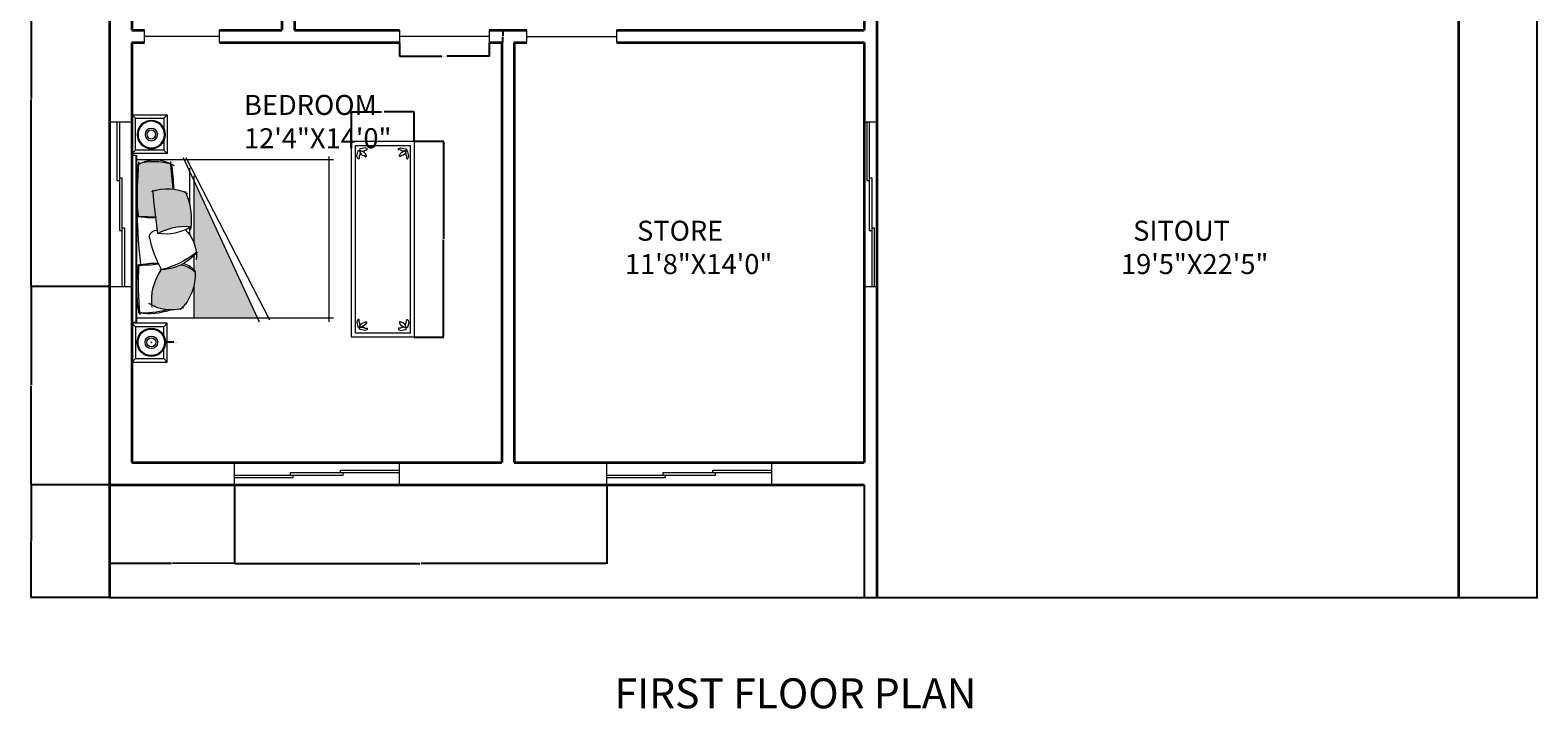
# Model space of a CAD drawing. Units: inches. Extents: x 1569 to 2779, y 1228 to 1844.
# Tile 5 of 6: x 2176 to 2779, y 1228 to 1500. Entities that reach past the tile are written whole.
import ezdxf

# ---------------------------------------------------------------- set-up
doc = ezdxf.new("R2010")
doc.units = ezdxf.units.IN
for name, color, linetype, lineweight in [('0.10', 252, 'Continuous', 9), ('0.15', 34, 'Continuous', 15), ('A-ANNO-DIMS', 2, 'Continuous', 18), ('A-ANNO-TEXT', 7, 'Continuous', 25), ('A-AREA-IDEN', 7, 'Continuous', 18), ('A-DOOR', 3, 'Continuous', 20), ('A-FLOR-EDGE', 7, 'Continuous', 25), ('A-FURN', 8, 'Continuous', 13), ('A-FURN-PATT', 116, 'Continuous', 9), ('A-GLAZ', 5, 'Continuous', 18), ('A-WALL', 7, 'Continuous', 35)]:
    doc.layers.add(name, color=color, linetype=linetype, lineweight=lineweight)
doc.styles.get("Standard").update_dxf_attribs({"font": 'arial.ttf'})
doc.dimstyles.get("Standard").update_dxf_attribs({"dimtxt": 0.18, "dimasz": 0.18, "dimexe": 0.18, "dimexo": 0.0625, "dimgap": 0.09, "dimtad": 0, "dimtih": 1, "dimtoh": 1, "dimdec": 4, "dimzin": 0, "dimdsep": 46, "dimtxsty": 'Standard', "dimcen": 0.09, "dimadec": 0, "dimazin": 0, "dimtfac": 1, "dimtdec": 4, "dimtofl": 0, "dimtmove": 0, "dimatfit": 3, "dimfxl": 1, "dimtolj": 1, "dimtzin": 0, "dimarcsym": 0})

# ---------------------------------------------------------------- blocks, each defined once
blk = doc.blocks.new('camita')
at = {"layer": '0.10'}
for p, q in [((-0.85, -0.045), (0.85, -0.045)), ((-0.805, -0.045), (-0.805, -2.048)), ((0.805, -0.045), (0.805, -2.048)), ((-0.827, -0.521), (0.846, -1.293)), ((-0.827, -0.548), (0.824, -1.399)), ((-0.716, -0.585), (-0.355, -0.585)), ((-0.114, -0.585), (-0.049, -0.585)), ((-0.638, -0.63), (0.043, -0.63)), ((0.175, -0.63), (0.318, -0.63)), ((0.474, -0.63), (0.805, -0.63)), ((-0.835, -2), (0.846, -2))]:
    blk.add_line(p, q, dxfattribs=at)
blk.add_lwpolyline([(-0.85, -0.041), (0.85, -0.041), (0.85, 0), (-0.85, 0)], close=True, dxfattribs=at)
for centre, radius, start, end in [((-0.457, -0.236), 0.344, 147.51, 213.8336), ((-0.2, -0.227), 0.586, 163.9263, 197.1409), ((-0.364, -5.846), 5.791, 83.8073, 94.1211), ((-0.51, -1.723), 1.678, 80.1255, 98.6619), ((2.353, -0.053), 2.58, 180.1063, 184.3854), ((-1.544, -0.245), 1.333, 359.9394, 7.5533), ((1.581, -0.289), 1.335, 170.3802, 178.9914), ((-1.44, -0.061), 1.712, 352.9291, 0.3959), ((0.452, -3.067), 3, 83.9026, 93.6759), ((0.486, -1.629), 1.578, 80.1602, 98.06), ((0.029, -0.138), 0.726, 342.5841, 6.0048), ((0.133, -0.17), 0.631, 339.923, 8.7433), ((-0.054, -0.363), 0.454, 159.3026, 206.5026), ((-1.33, -9.675), 9.499, 82.2708, 84.9399), ((0.458, -0.545), 0.584, 151.0456, 184.1497), ((-0.534, -0.339), 0.487, 327.2644, 9.0473), ((-0.007, -0.258), 0.0828, 100.018, 179.736), ((-0.293, -1.438), 1.29, 61.9749, 77.8435), ((-0.199, -0.274), 0.516, 310.7395, 359.0576), ((-0.567, -0.087), 0.906, 321.6953, 346.4626), ((0.627, -0.752), 0.551, 82.9691, 124.6739), ((0.32, -0.394), 0.404, 341.4524, 33.4512), ((-1.867, -14.986), 14.632, 84.6597, 85.7516), ((-0.46, 1.486), 1.909, 260.953, 268.6517), ((-0.2, 0.064), 0.667, 244.7809, 279.0606), ((0.179, -0.272), 0.383, 224.5284, 275.2229), ((0.438, -0.483), 0.19, 193.6849, 236.7035), ((0.571, -0.432), 0.315, 192.9388, 221.9636), ((0.361, -0.133), 0.51, 267.2589, 315.2997)]:
    blk.add_arc(centre, radius, start, end, dxfattribs=at)
blk = doc.blocks.new('VELADOR')
at = {"layer": '0.15'}
for p, q in [((-0.248, 0), (-0.203, -0.045)), ((0.248, 0), (0.202, -0.045)), ((-0.203, -0.405), (-0.248, -0.45)), ((0.248, -0.45), (0.202, -0.405))]:
    blk.add_line(p, q, dxfattribs=at)
blk.add_lwpolyline([(-0.248, 0), (-0.248, -0.45), (0.248, -0.45), (0.248, 0)], close=True, dxfattribs=at)
blk.add_lwpolyline([(0.092, -0.405), (0.202, -0.405), (0.202, -0.045), (-0.203, -0.045), (-0.203, -0.405), (-0.082, -0.405)], dxfattribs=at)
for radius in [0.18, 0.169, 0.0788, 0.0563]:
    blk.add_circle((0.005, -0.247), radius, dxfattribs=at)
blk = doc.blocks.new('carpet-7')
at = {"color": 0, "linetype": 'ByBlock'}
for p, q in [((-1.022, 0), (0, 0)), ((0, 0), (0, -0.54)), ((-1.694, -0.54), (-1.694, 0)), ((-1.694, 0), (-1.022, 0)), ((-1.658, -0.508), (-1.658, -0.032)), ((-1.658, -0.032), (-0.036, -0.032)), ((-1.636, -0.116), (-1.634, -0.103)), ((-1.629, -0.131), (-1.636, -0.116)), ((-1.634, -0.103), (-1.63, -0.09)), ((-1.63, -0.09), (-1.626, -0.07)), ((-1.626, -0.07), (-1.617, -0.069)), ((-1.617, -0.069), (-1.612, -0.072)), ((-1.615, -0.116), (-1.617, -0.134)), ((-1.608, -0.102), (-1.615, -0.116)), ((-1.611, -0.056), (-1.612, -0.064)), ((-1.612, -0.064), (-1.609, -0.068)), ((-1.612, -0.072), (-1.606, -0.089)), ((-1.59, -0.052), (-1.611, -0.056)), ((-1.609, -0.068), (-1.591, -0.073)), ((-1.609, -0.079), (-1.603, -0.072)), ((-1.599, -0.096), (-1.609, -0.079)), ((-1.606, -0.089), (-1.608, -0.102)), ((-1.603, -0.072), (-1.597, -0.072)), ((-1.593, -0.108), (-1.599, -0.096)), ((-1.597, -0.072), (-1.581, -0.081)), ((-1.585, -0.12), (-1.593, -0.108)), ((-1.591, -0.073), (-1.576, -0.072)), ((-1.575, -0.049), (-1.59, -0.052)), ((-1.569, -0.127), (-1.585, -0.12)), ((-1.581, -0.081), (-1.573, -0.092)), ((-1.576, -0.072), (-1.561, -0.066)), ((-1.561, -0.046), (-1.575, -0.049)), ((-1.573, -0.092), (-1.568, -0.107)), ((-1.563, -0.127), (-1.569, -0.127)), ((-1.568, -0.107), (-1.557, -0.123)), ((-1.557, -0.123), (-1.563, -0.127)), ((-1.544, -0.053), (-1.561, -0.046)), ((-1.561, -0.066), (-1.54, -0.064)), ((-1.54, -0.056), (-1.544, -0.053)), ((-1.54, -0.064), (-1.54, -0.056)), ((-0.151, -0.056), (-0.148, -0.053)), ((-0.151, -0.064), (-0.151, -0.056)), ((-0.131, -0.066), (-0.151, -0.064)), ((-0.148, -0.053), (-0.131, -0.046)), ((-0.124, -0.107), (-0.134, -0.123)), ((-0.134, -0.123), (-0.128, -0.127)), ((-0.131, -0.046), (-0.116, -0.049)), ((-0.115, -0.072), (-0.131, -0.066)), ((-0.128, -0.127), (-0.122, -0.127)), ((-0.119, -0.092), (-0.124, -0.107)), ((-0.122, -0.127), (-0.107, -0.12)), ((-0.11, -0.081), (-0.119, -0.092)), ((-0.116, -0.049), (-0.102, -0.052)), ((-0.101, -0.073), (-0.115, -0.072)), ((-0.095, -0.072), (-0.11, -0.081)), ((-0.107, -0.12), (-0.098, -0.108)), ((-0.102, -0.052), (-0.08, -0.056)), ((-0.083, -0.068), (-0.101, -0.073)), ((-0.098, -0.108), (-0.092, -0.096)), ((-0.089, -0.072), (-0.095, -0.072)), ((-0.092, -0.096), (-0.083, -0.079)), ((-0.083, -0.079), (-0.089, -0.072)), ((-0.079, -0.072), (-0.085, -0.089)), ((-0.085, -0.089), (-0.084, -0.102)), ((-0.084, -0.102), (-0.077, -0.116)), ((-0.079, -0.064), (-0.083, -0.068)), ((-0.08, -0.056), (-0.079, -0.064)), ((-0.074, -0.069), (-0.079, -0.072)), ((-0.077, -0.116), (-0.074, -0.134)), ((-0.066, -0.07), (-0.074, -0.069)), ((-0.061, -0.09), (-0.066, -0.07)), ((-0.062, -0.131), (-0.055, -0.116)), ((-0.058, -0.103), (-0.061, -0.09)), ((-0.055, -0.116), (-0.058, -0.103)), ((-0.036, -0.032), (-0.036, -0.508)), ((-1.626, -0.134), (-1.629, -0.131)), ((-1.617, -0.134), (-1.626, -0.134)), ((-0.074, -0.134), (-0.066, -0.134)), ((-0.066, -0.134), (-0.062, -0.131)), ((-1.658, -0.508), (-0.036, -0.508)), ((-1.629, -0.409), (-1.636, -0.424)), ((-1.636, -0.424), (-1.634, -0.437)), ((-1.634, -0.437), (-1.63, -0.45)), ((-1.63, -0.45), (-1.626, -0.47)), ((-1.626, -0.406), (-1.629, -0.409)), ((-1.617, -0.406), (-1.626, -0.406)), ((-1.626, -0.47), (-1.617, -0.471)), ((-1.615, -0.424), (-1.617, -0.406)), ((-1.617, -0.471), (-1.612, -0.468)), ((-1.608, -0.438), (-1.615, -0.424)), ((-1.612, -0.468), (-1.606, -0.451)), ((-1.612, -0.476), (-1.609, -0.472)), ((-1.611, -0.484), (-1.612, -0.476)), ((-1.59, -0.488), (-1.611, -0.484)), ((-1.599, -0.444), (-1.609, -0.461)), ((-1.609, -0.461), (-1.603, -0.468)), ((-1.609, -0.472), (-1.591, -0.467)), ((-1.606, -0.451), (-1.608, -0.438)), ((-1.603, -0.468), (-1.597, -0.468)), ((-1.593, -0.432), (-1.599, -0.444)), ((-1.597, -0.468), (-1.581, -0.459)), ((-1.585, -0.42), (-1.593, -0.432)), ((-1.591, -0.467), (-1.576, -0.468)), ((-1.575, -0.491), (-1.59, -0.488)), ((-1.569, -0.413), (-1.585, -0.42)), ((-1.581, -0.459), (-1.573, -0.448)), ((-1.576, -0.468), (-1.561, -0.474)), ((-1.561, -0.494), (-1.575, -0.491)), ((-1.573, -0.448), (-1.568, -0.433)), ((-1.563, -0.413), (-1.569, -0.413)), ((-1.568, -0.433), (-1.557, -0.417)), ((-1.557, -0.417), (-1.563, -0.413)), ((-1.561, -0.474), (-1.54, -0.476)), ((-1.544, -0.487), (-1.561, -0.494)), ((-1.54, -0.484), (-1.544, -0.487)), ((-1.54, -0.476), (-1.54, -0.484)), ((-0.131, -0.474), (-0.151, -0.476)), ((-0.151, -0.476), (-0.151, -0.484)), ((-0.151, -0.484), (-0.148, -0.487)), ((-0.148, -0.487), (-0.131, -0.494)), ((-0.134, -0.417), (-0.128, -0.413)), ((-0.124, -0.433), (-0.134, -0.417)), ((-0.115, -0.468), (-0.131, -0.474)), ((-0.131, -0.494), (-0.116, -0.491)), ((-0.128, -0.413), (-0.122, -0.413)), ((-0.119, -0.448), (-0.124, -0.433)), ((-0.122, -0.413), (-0.107, -0.42)), ((-0.11, -0.459), (-0.119, -0.448)), ((-0.116, -0.491), (-0.102, -0.488)), ((-0.101, -0.467), (-0.115, -0.468)), ((-0.095, -0.468), (-0.11, -0.459)), ((-0.107, -0.42), (-0.098, -0.432)), ((-0.102, -0.488), (-0.08, -0.484)), ((-0.083, -0.472), (-0.101, -0.467)), ((-0.098, -0.432), (-0.092, -0.444)), ((-0.089, -0.468), (-0.095, -0.468)), ((-0.092, -0.444), (-0.083, -0.461)), ((-0.083, -0.461), (-0.089, -0.468)), ((-0.085, -0.451), (-0.084, -0.438)), ((-0.079, -0.468), (-0.085, -0.451)), ((-0.084, -0.438), (-0.077, -0.424)), ((-0.079, -0.476), (-0.083, -0.472)), ((-0.08, -0.484), (-0.079, -0.476)), ((-0.074, -0.471), (-0.079, -0.468)), ((-0.077, -0.424), (-0.074, -0.406)), ((-0.074, -0.406), (-0.066, -0.406)), ((-0.066, -0.47), (-0.074, -0.471)), ((-0.066, -0.406), (-0.062, -0.409)), ((-0.061, -0.45), (-0.066, -0.47)), ((-0.062, -0.409), (-0.055, -0.424)), ((-0.058, -0.437), (-0.061, -0.45)), ((-0.055, -0.424), (-0.058, -0.437)), ((0, -0.54), (-1.694, -0.54))]:
    blk.add_line(p, q, dxfattribs=at)
blk = doc.blocks.new('WIN-66IN')
for p, q in [((0, 0), (0, 9)), ((66, 0), (66, 9)), ((0, 4), (43.5, 4)), ((0, 3), (23.5, 3)), ((22.5, 5), (66, 5)), ((22.5, 4), (22.5, 5)), ((23.5, 3), (23.5, 4)), ((42.5, 6), (66, 6)), ((42.5, 5), (42.5, 6)), ((43.5, 4), (43.5, 5))]:
    blk.add_line(p, q)
blk = doc.blocks.new('DOOR-30IN')
for p, q in [((0, 5), (0, 0)), ((0, 2.5), (30, 2.5)), ((30, 5), (30, 0))]:
    blk.add_line(p, q)
blk = doc.blocks.new('DOOR-36IN')
for p, q in [((0, 5), (0, 0)), ((36, 2.5), (0, 2.5)), ((36, 5), (36, 0))]:
    blk.add_line(p, q)
blk = doc.blocks.new('*D21')
at = {"layer": 'A-ANNO-DIMS', "color": 0, "lineweight": -2, "transparency": 16777216}
for p, q in [((2323.35, 1494.82), (2323.35, 1489.3)), ((2359.35, 1494.82), (2359.35, 1489.3)), ((2323.53, 1489.48), (2340.42, 1489.48)), ((2359.17, 1489.48), (2342.29, 1489.48))]:
    blk.add_line(p, q, dxfattribs=at)
at = {"layer": 'A-ANNO-DIMS', "color": 0, "transparency": 16777216}
for points in [[(2323.53, 1489.51), (2323.53, 1489.45), (2323.35, 1489.48)], [(2359.17, 1489.51), (2359.17, 1489.45), (2359.35, 1489.48)]]:
    blk.add_solid(points, dxfattribs=at)
at = {"layer": 'Defpoints', "color": 0, "transparency": 16777216}
for p in [(2323.35, 1494.88), (2359.35, 1494.88), (2359.35, 1489.48)]:
    blk.add_point(p, dxfattribs=at)
at = {"layer": 'A-ANNO-DIMS', "color": 0, "transparency": 16777216, "insert": (2341.35, 1489.48), "char_height": 0.18, "attachment_point": 5}
blk.add_mtext('\\A1;DOOR 36 TYP.', dxfattribs=at)
blk = doc.blocks.new('*D22')
at = {"layer": 'A-ANNO-DIMS', "color": 0, "lineweight": -2, "transparency": 16777216}
for p, q in [((2359.41, 1499.88), (2364.93, 1499.88)), ((2364.75, 1499.7), (2364.75, 1497.56)), ((2364.75, 1495.06), (2364.75, 1497.2)), ((2359.41, 1494.88), (2364.93, 1494.88))]:
    blk.add_line(p, q, dxfattribs=at)
at = {"layer": 'A-ANNO-DIMS', "color": 0, "transparency": 16777216}
for points in [[(2364.72, 1499.7), (2364.78, 1499.7), (2364.75, 1499.88)], [(2364.72, 1495.06), (2364.78, 1495.06), (2364.75, 1494.88)]]:
    blk.add_solid(points, dxfattribs=at)
at = {"layer": 'Defpoints', "color": 0, "transparency": 16777216}
for p in [(2359.35, 1499.88), (2364.75, 1499.88), (2359.35, 1494.88)]:
    blk.add_point(p, dxfattribs=at)
at = {"layer": 'A-ANNO-DIMS', "color": 0, "transparency": 16777216, "insert": (2364.75, 1497.38), "char_height": 0.18, "attachment_point": 5}
blk.add_mtext('\\A1;5 TYP.', dxfattribs=at)
blk = doc.blocks.new('*D35')
at = {"layer": 'A-ANNO-DIMS', "color": 0, "lineweight": -2, "transparency": 16777216}
for p, q in [((2329.32, 1455.4), (2341.19, 1455.4)), ((2341.01, 1455.22), (2341.01, 1416.38)), ((2341.01, 1377.19), (2341.01, 1416.02)), ((2329.32, 1377.01), (2341.19, 1377.01))]:
    blk.add_line(p, q, dxfattribs=at)
at = {"layer": 'A-ANNO-DIMS', "color": 0, "transparency": 16777216}
for points in [[(2340.98, 1455.22), (2341.04, 1455.22), (2341.01, 1455.4)], [(2340.98, 1377.19), (2341.04, 1377.19), (2341.01, 1377.01)]]:
    blk.add_solid(points, dxfattribs=at)
at = {"layer": 'Defpoints', "color": 0, "transparency": 16777216}
for p in [(2329.26, 1455.4), (2341.01, 1455.4), (2329.26, 1377.01)]:
    blk.add_point(p, dxfattribs=at)
at = {"layer": 'A-ANNO-DIMS', "color": 0, "transparency": 16777216, "insert": (2341.01, 1416.2), "char_height": 0.18, "attachment_point": 5}
blk.add_mtext('\\A1;RUG 78 TYP.', dxfattribs=at)
blk = doc.blocks.new('*D36')
at = {"layer": 'A-ANNO-DIMS', "color": 0, "lineweight": -2, "transparency": 16777216}
for p, q in [((2304.27, 1455.46), (2304.27, 1467.33)), ((2304.45, 1467.15), (2316.23, 1467.15)), ((2329.08, 1467.15), (2317.29, 1467.15)), ((2329.26, 1455.46), (2329.26, 1467.33))]:
    blk.add_line(p, q, dxfattribs=at)
at = {"layer": 'A-ANNO-DIMS', "color": 0, "transparency": 16777216}
for points in [[(2304.45, 1467.18), (2304.45, 1467.12), (2304.27, 1467.15)], [(2329.08, 1467.18), (2329.08, 1467.12), (2329.26, 1467.15)]]:
    blk.add_solid(points, dxfattribs=at)
at = {"layer": 'Defpoints', "color": 0, "transparency": 16777216}
for p in [(2304.27, 1467.15), (2304.27, 1455.4), (2329.26, 1455.4)]:
    blk.add_point(p, dxfattribs=at)
at = {"layer": 'A-ANNO-DIMS', "color": 0, "transparency": 16777216, "insert": (2316.76, 1467.15), "char_height": 0.18, "attachment_point": 5}
blk.add_mtext('\\A1;25 TYP.', dxfattribs=at)
blk = doc.blocks.new('*D51')
at = {"layer": 'A-ANNO-DIMS', "color": 0, "lineweight": -2, "transparency": 16777216}
for p, q in [((2747.41, 1812.88), (2778.88, 1812.88)), ((2778.7, 1812.7), (2778.7, 1543.06)), ((2778.7, 1273.06), (2778.7, 1542.7)), ((2747.41, 1272.88), (2778.88, 1272.88))]:
    blk.add_line(p, q, dxfattribs=at)
at = {"layer": 'A-ANNO-DIMS', "color": 0, "transparency": 16777216}
for points in [[(2778.67, 1812.7), (2778.73, 1812.7), (2778.7, 1812.88)], [(2778.67, 1273.06), (2778.73, 1273.06), (2778.7, 1272.88)]]:
    blk.add_solid(points, dxfattribs=at)
at = {"layer": 'Defpoints', "color": 0, "transparency": 16777216}
for p in [(2747.35, 1812.88), (2778.7, 1812.88), (2747.35, 1272.88)]:
    blk.add_point(p, dxfattribs=at)
at = {"layer": 'A-ANNO-DIMS', "color": 0, "transparency": 16777216, "insert": (2778.7, 1542.88), "char_height": 0.18, "attachment_point": 5}
blk.add_mtext('\\A1;540', dxfattribs=at)
blk = doc.blocks.new('*D52')
at = {"layer": 'A-ANNO-DIMS', "color": 0, "lineweight": -2, "transparency": 16777216}
for p, q in [((2207.29, 1317.88), (2175.82, 1317.88)), ((2176, 1317.7), (2176, 1295.56)), ((2176, 1273.06), (2176, 1295.2)), ((2207.29, 1272.88), (2175.82, 1272.88))]:
    blk.add_line(p, q, dxfattribs=at)
at = {"layer": 'A-ANNO-DIMS', "color": 0, "transparency": 16777216}
for points in [[(2175.97, 1317.7), (2176.03, 1317.7), (2176, 1317.88)], [(2175.97, 1273.06), (2176.03, 1273.06), (2176, 1272.88)]]:
    blk.add_solid(points, dxfattribs=at)
at = {"layer": 'Defpoints', "color": 0, "transparency": 16777216}
for p in [(2176, 1317.88), (2207.35, 1317.88), (2207.35, 1272.88)]:
    blk.add_point(p, dxfattribs=at)
at = {"layer": 'A-ANNO-DIMS', "color": 0, "transparency": 16777216, "insert": (2176, 1295.38), "char_height": 0.18, "attachment_point": 5}
blk.add_mtext('\\A1;45', dxfattribs=at)
blk = doc.blocks.new('*D71')
at = {"layer": 'A-ANNO-DIMS', "color": 0, "lineweight": -2, "transparency": 16777216}
for p, q in [((2207.35, 1317.82), (2207.34, 1286.35)), ((2257.35, 1317.8), (2257.34, 1286.33)), ((2207.52, 1286.53), (2232.12, 1286.52)), ((2257.16, 1286.51), (2232.56, 1286.52))]:
    blk.add_line(p, q, dxfattribs=at)
at = {"layer": 'A-ANNO-DIMS', "color": 0, "transparency": 16777216}
for points in [[(2207.52, 1286.56), (2207.52, 1286.5), (2207.34, 1286.53)], [(2257.16, 1286.54), (2257.16, 1286.48), (2257.34, 1286.51)]]:
    blk.add_solid(points, dxfattribs=at)
at = {"layer": 'Defpoints', "color": 0, "transparency": 16777216}
for p in [(2207.35, 1317.88), (2257.35, 1317.86), (2207.34, 1286.53)]:
    blk.add_point(p, dxfattribs=at)
at = {"layer": 'A-ANNO-DIMS', "color": 0, "transparency": 16777216, "insert": (2232.34, 1286.52), "char_height": 0.18, "attachment_point": 5}
blk.add_mtext('\\A1;50', dxfattribs=at)
blk = doc.blocks.new('*D72')
at = {"layer": 'A-ANNO-DIMS', "color": 0, "lineweight": -2, "transparency": 16777216}
for p, q in [((2257.35, 1317.8), (2257.35, 1286.33)), ((2406.35, 1317.8), (2406.35, 1286.33)), ((2257.53, 1286.51), (2331.57, 1286.51)), ((2406.17, 1286.51), (2332.13, 1286.51))]:
    blk.add_line(p, q, dxfattribs=at)
at = {"layer": 'A-ANNO-DIMS', "color": 0, "transparency": 16777216}
for points in [[(2257.53, 1286.54), (2257.53, 1286.48), (2257.35, 1286.51)], [(2406.17, 1286.54), (2406.17, 1286.48), (2406.35, 1286.51)]]:
    blk.add_solid(points, dxfattribs=at)
at = {"layer": 'Defpoints', "color": 0, "transparency": 16777216}
for p in [(2257.35, 1317.86), (2406.35, 1317.86), (2257.35, 1286.51)]:
    blk.add_point(p, dxfattribs=at)
at = {"layer": 'A-ANNO-DIMS', "color": 0, "transparency": 16777216, "insert": (2331.85, 1286.51), "char_height": 0.18, "attachment_point": 5}
blk.add_mtext('\\A1;149', dxfattribs=at)
blk = doc.blocks.new('*D73')
at = {"layer": 'A-ANNO-DIMS', "color": 0, "lineweight": -2, "transparency": 16777216}
for p, q in [((2207.29, 1397.25), (2175.82, 1397.25)), ((2176, 1397.07), (2176, 1357.75)), ((2176, 1318.06), (2176, 1357.38)), ((2207.29, 1317.88), (2175.82, 1317.88))]:
    blk.add_line(p, q, dxfattribs=at)
at = {"layer": 'A-ANNO-DIMS', "color": 0, "transparency": 16777216}
for points in [[(2175.97, 1397.07), (2176.03, 1397.07), (2176, 1397.25)], [(2175.97, 1318.06), (2176.03, 1318.06), (2176, 1317.88)]]:
    blk.add_solid(points, dxfattribs=at)
at = {"layer": 'Defpoints', "color": 0, "transparency": 16777216}
for p in [(2176, 1397.25), (2207.35, 1397.25), (2207.35, 1317.88)]:
    blk.add_point(p, dxfattribs=at)
at = {"layer": 'A-ANNO-DIMS', "color": 0, "transparency": 16777216, "insert": (2176, 1357.56), "char_height": 0.18, "attachment_point": 5}
blk.add_mtext('\\A1;79.37', dxfattribs=at)
blk = doc.blocks.new('*D74')
at = {"layer": 'A-ANNO-DIMS', "color": 0, "lineweight": -2, "transparency": 16777216}
for p, q in [((2207.29, 1547.38), (2175.82, 1547.38)), ((2176, 1547.2), (2176, 1472.5)), ((2176, 1397.43), (2176, 1472.13)), ((2207.29, 1397.25), (2175.82, 1397.25))]:
    blk.add_line(p, q, dxfattribs=at)
at = {"layer": 'A-ANNO-DIMS', "color": 0, "transparency": 16777216}
for points in [[(2175.97, 1547.2), (2176.03, 1547.2), (2176, 1547.38)], [(2175.97, 1397.43), (2176.03, 1397.43), (2176, 1397.25)]]:
    blk.add_solid(points, dxfattribs=at)
at = {"layer": 'Defpoints', "color": 0, "transparency": 16777216}
for p in [(2176, 1547.38), (2207.35, 1547.38), (2207.35, 1397.25)]:
    blk.add_point(p, dxfattribs=at)
at = {"layer": 'A-ANNO-DIMS', "color": 0, "transparency": 16777216, "insert": (2176, 1472.31), "char_height": 0.18, "attachment_point": 5}
blk.add_mtext('\\A1;150.13', dxfattribs=at)
blk = doc.blocks.new('*D87')
at = {"layer": 'A-ANNO-DIMS', "color": 0, "lineweight": -2, "transparency": 16777216}
for p, q in [((2224.03, 1374.96), (2224.21, 1374.96)), ((2224.12, 1374.87), (2224.12, 1375.05)), ((2233.17, 1374.96), (2229.96, 1374.96))]:
    blk.add_line(p, q, dxfattribs=at)
at = {"layer": 'A-ANNO-DIMS', "color": 0, "transparency": 16777216}
blk.add_solid([(2229.96, 1374.99), (2229.96, 1374.93), (2229.78, 1374.96)], dxfattribs=at)
at = {"layer": 'Defpoints', "color": 0, "transparency": 16777216}
for p in [(2218.47, 1374.96), (2229.78, 1374.96)]:
    blk.add_point(p, dxfattribs=at)
at = {"layer": 'A-ANNO-DIMS', "color": 0, "transparency": 16777216, "insert": (2233.83, 1374.96), "char_height": 0.18, "attachment_point": 5}
blk.add_mtext('\\A1;3X ∅11.31', dxfattribs=at)

msp = doc.modelspace()

# ---------------------------------------------------------------- hatches: boundary and pattern name
at = {"layer": 'A-FURN-PATT'}
h = msp.add_hatch(color=256, dxfattribs=at)
h.dxf.hatch_style = 1
h.paths.add_polyline_path([(2231.9265, 1446.3888, 0.14222248), (2219.0532, 1446.5152, 0.02322168), (2218.5711, 1425.3523, -0.01794435), (2225.8563, 1425.0816, -0.00696723), (2224.7826, 1435.4488, -0.11389129), (2232.7792, 1436.3149, -0.00438694)])
h.paths.add_polyline_path([(2241.1575, 1414.7086, -0.16677621), (2241.4673, 1404.9309, -0.09017801), (2241.1575, 1397.7575), (2241.1575, 1384.7212), (2266.5173, 1384.7212), (2241.1575, 1439.683)])
h = msp.add_hatch(color=256, dxfattribs=at)
h.dxf.hatch_style = 1
h.paths.add_polyline_path([(2237.8675, 1434.9727, 0.18953567), (2224.7889, 1435.4952, 0.01140771), (2226.6975, 1418.5384, -0.1503613), (2239.9372, 1421.3169, 0.13377603)])
h.paths.add_polyline_path([(2224.363, 1389.8217, 0.1949524), (2236.255, 1388.541, 0.20255928), (2241.6379, 1403.2024, 0.12732633), (2236.1303, 1406.0635, -0.10404536), (2228.0277, 1403.9922, 0.17383481)])

# ---------------------------------------------------------------- linework, layer by layer
at = {"layer": 'A-FLOR-EDGE'}
for p, q in [((2509.3512, 1317.8785), (2509.3512, 1272.8785)), ((2207.3512, 1272.8785), (2747.3512, 1272.8785))]:
    msp.add_line(p, q, dxfattribs=at)
at = {"layer": 'A-GLAZ'}
for p, q in [((2509.3512, 1463.2502), (2514.3512, 1463.2502)), ((2510.3512, 1463.2502), (2510.3512, 1439.7502)), ((2511.3512, 1463.2502), (2511.3512, 1419.7502)), ((2510.3512, 1439.7502), (2511.3512, 1439.7502)), ((2511.3512, 1440.7502), (2512.3512, 1440.7502)), ((2512.3512, 1440.7502), (2512.3512, 1397.2502)), ((2511.3512, 1419.7502), (2512.3512, 1419.7502)), ((2512.3512, 1420.7502), (2513.3512, 1420.7502)), ((2513.3512, 1420.7502), (2513.3512, 1397.2502)), ((2509.3512, 1397.2502), (2514.3512, 1397.2502))]:
    msp.add_line(p, q, dxfattribs=at)
at = {"layer": 'A-WALL'}
for p, q in [((2207.3512, 1812.8785), (2207.3512, 1272.8785)), ((2747.3512, 1272.8785), (2747.3512, 1812.8785)), ((2216.3512, 1618.8785), (2216.3512, 1499.8785)), ((2276.3512, 1618.8785), (2276.3512, 1499.8785)), ((2281.3512, 1618.8785), (2281.3512, 1499.8785)), ((2509.3512, 1546.8785), (2509.3512, 1499.8785)), ((2514.3512, 1546.8785), (2514.3512, 1272.8785)), ((2216.3512, 1499.8785), (2221.3512, 1499.8785)), ((2251.3512, 1499.8785), (2276.3512, 1499.8785)), ((2281.3512, 1499.8785), (2323.3512, 1499.8785)), ((2359.3512, 1499.8785), (2374.3512, 1499.8785)), ((2410.3512, 1499.8785), (2509.3512, 1499.8785)), ((2216.3512, 1494.8785), (2221.3512, 1494.8785)), ((2216.3512, 1494.8785), (2216.3512, 1326.8785)), ((2251.3512, 1494.8785), (2323.3512, 1494.8785)), ((2359.3512, 1494.8785), (2364.3512, 1494.8785)), ((2364.3512, 1494.8785), (2364.3512, 1326.8785)), ((2369.3512, 1494.8785), (2369.3512, 1326.8785)), ((2369.3512, 1494.8785), (2374.3512, 1494.8785)), ((2410.3512, 1494.8785), (2509.3512, 1494.8785)), ((2509.3512, 1494.8785), (2509.3512, 1326.8785)), ((2216.3512, 1326.8785), (2364.3512, 1326.8785)), ((2369.3512, 1326.8785), (2509.3512, 1326.8785)), ((2207.3512, 1317.8785), (2509.3512, 1317.8785))]:
    msp.add_line(p, q, dxfattribs=at)

# ---------------------------------------------------------------- block references
at = {"layer": 'A-DOOR', "rotation": 180}
for name, p in [('DOOR-30IN', (2251.3512, 1499.8785)), ('DOOR-36IN', (2410.3512, 1499.8785))]:
    msp.add_blockref(name, p, dxfattribs=at)
at = {"layer": 'A-DOOR'}
msp.add_blockref('DOOR-36IN', (2323.3512, 1494.8785), dxfattribs=at)
at = {"layer": 'A-FURN'}
for name, p, xscale, yscale, zscale, rotation in [('VELADOR', (2216.3512, 1458.2493), -31.41542173157097, 31.41542173157097, 31.41542173157097, 90), ('carpet-7', (2304.2674, 1455.3962), 46.2750735389499, 46.2750735389499, 46.2750735389499, 90), ('camita', (2216.3512, 1416.418), -39.375, 39.375, 39.375, 90), ('VELADOR', (2216.3512, 1374.7999), 31.41542173157097, 31.41542173157097, 31.41542173157097, 90.00000000000011)]:
    msp.add_blockref(name, p, dxfattribs=dict(at, xscale=xscale, yscale=yscale, zscale=zscale, rotation=rotation))
at = {"layer": 'A-GLAZ', "rotation": 269.9999999999998}
msp.add_blockref('WIN-66IN', (2207.3512, 1463.2502), dxfattribs=at)
at = {"layer": 'A-GLAZ'}
for p in [(2257.3512, 1317.863), (2406.3512, 1317.863)]:
    msp.add_blockref('WIN-66IN', p, dxfattribs=at)

# ---------------------------------------------------------------- texts
at = {"layer": 'A-ANNO-TEXT', "insert": (2409.4514, 1240.4981), "char_height": 12, "attachment_point": 1}
msp.add_mtext_dynamic_manual_height_columns('FIRST FLOOR PLAN', width=187.856256, gutter_width=12.5, heights=[0], dxfattribs=at)
at = {"layer": 'A-AREA-IDEN', "char_height": 8, "attachment_point": 1}
for s, insert in [('BEDROOM\\P12\'4"X14\'0"', (2261.1868, 1473.9559)), ('  STORE\\P11\'8"X14\'0"', (2413.5871, 1423.6131)), ('  SITOUT\\P19\'5"X22\'5"', (2612.0872, 1423.6131))]:
    msp.add_mtext_dynamic_manual_height_columns(s, width=101.861325, gutter_width=12.5, heights=[0], dxfattribs=dict(at, insert=insert))

# ---------------------------------------------------------------- dimensions: what is measured, and where the dimension line sits
at = {"layer": 'A-ANNO-DIMS'}
for base, p1, p2, angle, override, picture, middle in [((2778.7012, 1812.8785), (2747.3512, 1272.8785), (2747.3512, 1812.8785), 90, {"dimdec": 0, "dimlfac": 1, "dimrnd": 0, "dimzin": 0, "dimdsep": 46, "dimlunit": 2}, '*D51', (2778.7012, 1542.8785)), ((2176.0012, 1547.3785), (2207.3512, 1397.2502), (2207.3512, 1547.3785), 90, {"dimdec": 2, "dimlfac": 1, "dimrnd": 0, "dimzin": 0, "dimdsep": 46, "dimlunit": 2}, '*D74', (2176.0012, 1472.3143)), ((2176.0012, 1397.2502), (2207.3512, 1317.8785), (2207.3512, 1397.2502), 90, {"dimdec": 2, "dimlfac": 1, "dimrnd": 0, "dimzin": 0, "dimdsep": 46, "dimlunit": 2}, '*D73', (2176.0012, 1357.5643)), ((2176.0012, 1317.8785), (2207.3512, 1272.8785), (2207.3512, 1317.8785), 90, {"dimdec": 0, "dimlfac": 1, "dimrnd": 0, "dimzin": 0, "dimdsep": 46, "dimlunit": 2}, '*D52', (2176.0012, 1295.3785)), ((2207.3415, 1286.5285), (2257.3512, 1317.863), (2207.3512, 1317.8785), 179.9822905, {"dimdec": 0, "dimlfac": 1, "dimrnd": 0, "dimzin": 0, "dimdsep": 46, "dimlunit": 2}, '*D71', (2232.3415, 1286.5208)), ((2257.3512, 1286.513), (2406.3512, 1317.863), (2257.3512, 1317.863), 180, {"dimdec": 0, "dimlfac": 1, "dimrnd": 0, "dimzin": 0, "dimdsep": 46, "dimlunit": 2}, '*D72', (2331.8512, 1286.513))]:
    dim = msp.add_linear_dim(base=base, p1=p1, p2=p2, angle=angle, dimstyle='Standard', override=override, dxfattribs=at)
    dim.commit()
    dim.dimension.update_dxf_attribs({"geometry": picture, "text_midpoint": middle})
for base, p1, p2, angle, text, picture, middle in [((2364.7512, 1499.8785), (2359.3512, 1494.8785), (2359.3512, 1499.8785), 90, '<> TYP.', '*D22', (2364.7512, 1497.3785)), ((2304.2674, 1467.1545), (2329.2559, 1455.3962), (2304.2674, 1455.3962), 180, '<> TYP.', '*D36', (2316.7617, 1467.1545)), ((2341.0143, 1455.3962), (2329.2559, 1377.0071), (2329.2559, 1455.3962), 90, 'RUG <> TYP.', '*D35', (2341.0143, 1416.2016))]:
    dim = msp.add_linear_dim(base=base, p1=p1, p2=p2, angle=angle, text=text, dimstyle='Standard', override={"dimdec": 0, "dimlfac": 1, "dimrnd": 0, "dimzin": 0, "dimdsep": 46, "dimlunit": 2}, dxfattribs=at)
    dim.commit()
    dim.dimension.update_dxf_attribs({"geometry": picture, "text_midpoint": middle})
dim = msp.add_linear_dim(base=(2359.3512, 1489.4785), p1=(2323.3512, 1494.8785), p2=(2359.3512, 1494.8785), text='DOOR <> TYP.', dimstyle='Standard', override={"dimdec": 0, "dimlfac": 1, "dimrnd": 0, "dimzin": 0, "dimdsep": 46, "dimlunit": 2}, dxfattribs=at)
dim.commit()
dim.dimension.update_dxf_attribs({"geometry": '*D21', "text_midpoint": (2341.3512, 1489.4785)})
dim = msp.add_diameter_dim_2p(p1=(2218.4688, 1374.9624), p2=(2229.7784, 1374.962), text='3X <>', dimstyle='Standard', override={"dimdec": 2, "dimlfac": 1, "dimrnd": 0, "dimzin": 0, "dimdsep": 46, "dimlunit": 2}, dxfattribs=at)
dim.commit()
dim.dimension.update_dxf_attribs({"geometry": '*D87', "text_midpoint": (2233.1712, 1374.9619), "dimtype": 163})

doc.saveas('drawing.dxf')
